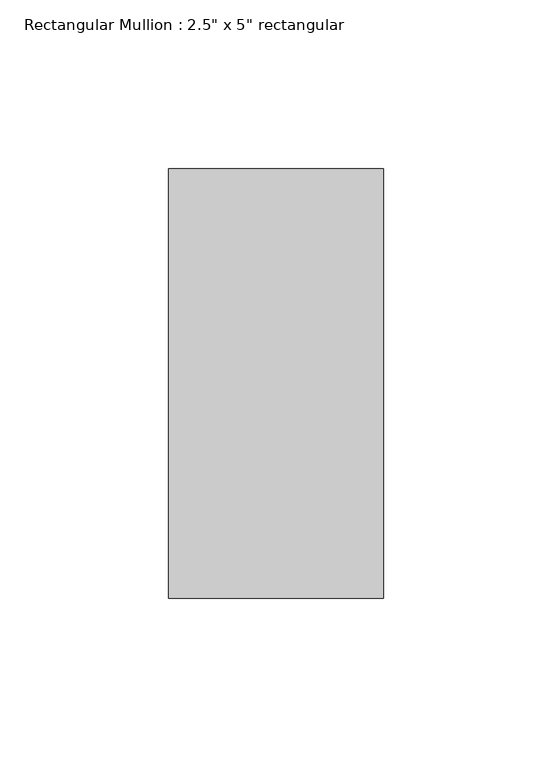
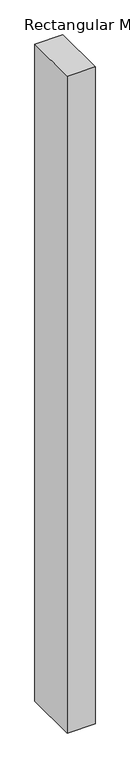
"""IFC4 building model written with IfcOpenShell, lengths in millimetres: member geometry."""

from ifc_helpers import new_model, si_unit, frame, origin, place, context, project, spatial, polyline, outline, extrude, source, transform, mapped, element, save


def member_971db604(model_context):
    return source(origin(), model_context, "Body", "SweptSolid", [
        extrude(outline(polyline([(0.0, 63.5), (0.0, -63.5), (-63.5, -63.5), (-63.5, 63.5), (0.0, 63.5)])), frame((0.0, 0.0, -1579.2479304), z_axis=(0.0, 0.0, 1.0), x_axis=(1.0, 0.0, 0.0)), (0.0, 0.0, 1.0), 1579.2479304),
    ])


if __name__ == "__main__":
    model = new_model("IFC4")
    model_context = context("Model", 3, world=origin())
    ifc_project = project(units=[si_unit("LENGTHUNIT", "METRE", prefix="MILLI")], contexts=[model_context])
    site = spatial("IfcSite", under=ifc_project)
    building = spatial("IfcBuilding", under=site)
    placement = place(None, origin())
    member_shape = member_971db604(model_context)
    element("IfcMember", 1, ObjectType="Rectangular Mullion : 2.5\" x 5\" rectangular", at=placement, inside=building, context=model_context, shape_type="MappedRepresentation", body=[
        mapped(member_shape, transform((0.0, 0.0, 0.0), x_axis=(1.0, 0.0, 0.0), y_axis=(0.0, 1.0, 0.0), z_axis=(0.0, 0.0, 1.0))),
    ])
    save(model, "model.ifc")

# Revit data of these elements
# Type "Rectangular Mullion : 2.5\" x 5\" rectangular"
#   built-in parameter 1007304 = 0.416667 (stored number, unit not read)
#   built-in parameter 1007301 = 0.104167 (stored number, unit not read)
#   built-in parameter 1007300 = 0.104167 (stored number, unit not read)
# Element 1 (IfcMember, "Rectangular Mullion : 2.5\" x 5\" rectangular")
#   Materials on its faces: "Aluminum"
# Materials
#   "Aluminum": class "Metal", colour RGB 247 247 247, transparency 0, Description = "Aluminum 6061", Cost = 0
